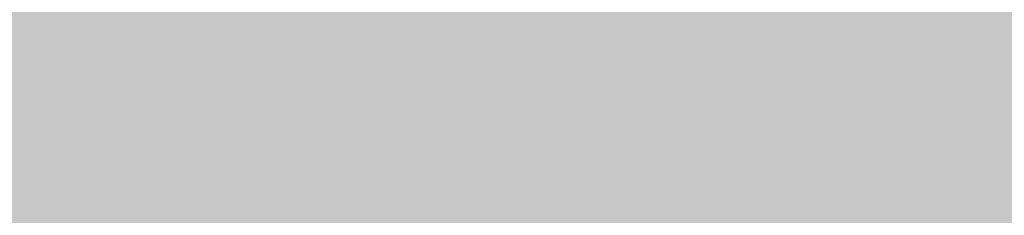
# Model space of a CAD drawing. Units: millimetres. Extents: x -22994 to 29398, y -19990 to 20176.
# Tile 92 of 135: x 229.428 to 230.597, y 83.564 to 83.796. Entities that reach past the tile are written whole.
import ezdxf
from ezdxf import colors
from ezdxf.entities.mleader import LeaderData, LeaderLine
from ezdxf.math import Vec2, Vec3

# ---------------------------------------------------------------- set-up
doc = ezdxf.new("R2010")
doc.units = ezdxf.units.MM
doc.header["$MEASUREMENT"] = 0
for name, color, linetype, lineweight in [('M-ANNO-TEXT', 7, 'Continuous', 25), ('M-DIMS', 2, 'Continuous', 18), ('M-EQPM-PATT', 7, 'Continuous', 18)]:
    doc.layers.add(name, color=color, linetype=linetype, lineweight=lineweight)
doc.styles.get("Standard").update_dxf_attribs({"font": 'arial.ttf'})
doc.dimstyles.get("Standard").update_dxf_attribs({"dimtxt": 0.18, "dimasz": 10000, "dimexe": 0.18, "dimexo": 0.0625, "dimgap": 0.09, "dimtad": 0, "dimtih": 1, "dimtoh": 1, "dimdec": 0, "dimzin": 0, "dimdsep": 46, "dimtxsty": 'Standard', "dimcen": 0.09, "dimadec": 0, "dimazin": 0, "dimtfac": 1, "dimtdec": 0, "dimtofl": 0, "dimtmove": 0, "dimatfit": 3, "dimfxl": 1, "dimtolj": 1, "dimtzin": 0, "dimlwd": 30, "dimarcsym": 0})

# ---------------------------------------------------------------- blocks, each defined once
blk = doc.blocks.new('*D2')
at = {"layer": 'Defpoints', "color": 0, "transparency": 16777216}
for p in [(6.6773, 10.2713), (290.852, 10.2713), (290.852, -5.0787)]:
    blk.add_point(p, dxfattribs=at)
at = {"layer": 'M-DIMS', "color": 0, "lineweight": -2, "transparency": 16777216}
for p, q in [((6.6773, 10.2088), (6.6773, -5.2587)), ((290.852, 10.2088), (290.852, -5.2587))]:
    blk.add_line(p, q, dxfattribs=at)
at = {"layer": 'M-DIMS', "color": 0, "lineweight": 30, "transparency": 16777216}
for p, q in [((-9993.3227, -5.0787), (-19993.3227, -5.0787)), ((10290.852, -5.0787), (20290.852, -5.0787))]:
    blk.add_line(p, q, dxfattribs=at)
at = {"layer": 'M-DIMS', "color": 0, "transparency": 16777216}
for points in [[(-9993.3227, 1661.5879), (-9993.3227, -1671.7454), (6.6773, -5.0787)], [(10290.852, 1661.5879), (10290.852, -1671.7454), (290.852, -5.0787)]]:
    blk.add_solid(points, dxfattribs=at)
at = {"layer": 'M-DIMS', "color": 0, "transparency": 16777216, "insert": (148.7647, -5.0787), "char_height": 0.18, "attachment_point": 5}
blk.add_mtext('\\A1;284.2', dxfattribs=at)
blk = doc.blocks.new('*D3')
at = {"layer": 'Defpoints', "color": 0, "transparency": 16777216}
for p in [(110.2647, 204.1654), (110.2647, 176.3662), (95.8327, 127.967)]:
    blk.add_point(p, dxfattribs=at)
at = {"layer": 'M-DIMS', "color": 0, "lineweight": -2, "transparency": 16777216}
for p, q in [((95.8327, 128.0295), (95.8327, 204.3454)), ((110.2647, 176.4287), (110.2647, 204.3454))]:
    blk.add_line(p, q, dxfattribs=at)
at = {"layer": 'M-DIMS', "color": 0, "lineweight": 30, "transparency": 16777216}
for p, q in [((-9904.1673, 204.1654), (-19904.1673, 204.1654)), ((10110.2647, 204.1654), (20110.2647, 204.1654))]:
    blk.add_line(p, q, dxfattribs=at)
at = {"layer": 'M-DIMS', "color": 0, "transparency": 16777216}
for points in [[(-9904.1673, 1870.8321), (-9904.1673, -1462.5013), (95.8327, 204.1654)], [(10110.2647, 1870.8321), (10110.2647, -1462.5013), (110.2647, 204.1654)]]:
    blk.add_solid(points, dxfattribs=at)
at = {"layer": 'M-DIMS', "color": 0, "transparency": 16777216, "insert": (103.0487, 204.1654), "char_height": 0.18, "attachment_point": 5}
blk.add_mtext('\\A1;14.432', dxfattribs=at)
blk = doc.blocks.new('*D4')
at = {"layer": 'Defpoints', "color": 0, "transparency": 16777216}
for p in [(116.2647, 204.1654), (110.2647, 176.3662), (116.2647, 176.3662)]:
    blk.add_point(p, dxfattribs=at)
at = {"layer": 'M-DIMS', "color": 0, "lineweight": -2, "transparency": 16777216}
for p, q in [((110.2647, 176.4287), (110.2647, 204.3454)), ((116.2647, 176.4287), (116.2647, 204.3454))]:
    blk.add_line(p, q, dxfattribs=at)
at = {"layer": 'M-DIMS', "color": 0, "lineweight": 30, "transparency": 16777216}
for p, q in [((-9889.7353, 204.1654), (-19889.7353, 204.1654)), ((10116.2647, 204.1654), (20116.2647, 204.1654))]:
    blk.add_line(p, q, dxfattribs=at)
at = {"layer": 'M-DIMS', "color": 0, "transparency": 16777216}
for points in [[(-9889.7353, 1870.8321), (-9889.7353, -1462.5013), (110.2647, 204.1654)], [(10116.2647, 1870.8321), (10116.2647, -1462.5013), (116.2647, 204.1654)]]:
    blk.add_solid(points, dxfattribs=at)
at = {"layer": 'M-DIMS', "color": 0, "transparency": 16777216, "insert": (113.2647, 204.1654), "char_height": 0.18, "attachment_point": 5}
blk.add_mtext('\\A1;6', dxfattribs=at)
blk = doc.blocks.new('*D5')
at = {"layer": 'Defpoints', "color": 0, "transparency": 16777216}
for p in [(181.2647, 204.1654), (116.2647, 176.3662), (181.2647, 176.3662)]:
    blk.add_point(p, dxfattribs=at)
at = {"layer": 'M-DIMS', "color": 0, "lineweight": -2, "transparency": 16777216}
for p, q in [((116.2647, 176.4287), (116.2647, 204.3454)), ((181.2647, 176.4287), (181.2647, 204.3454))]:
    blk.add_line(p, q, dxfattribs=at)
at = {"layer": 'M-DIMS', "color": 0, "lineweight": 30, "transparency": 16777216}
for p, q in [((-9883.7353, 204.1654), (-19883.7353, 204.1654)), ((10181.2647, 204.1654), (20181.2647, 204.1654))]:
    blk.add_line(p, q, dxfattribs=at)
at = {"layer": 'M-DIMS', "color": 0, "transparency": 16777216}
for points in [[(-9883.7353, 1870.8321), (-9883.7353, -1462.5013), (116.2647, 204.1654)], [(10181.2647, 1870.8321), (10181.2647, -1462.5013), (181.2647, 204.1654)]]:
    blk.add_solid(points, dxfattribs=at)
at = {"layer": 'M-DIMS', "color": 0, "transparency": 16777216, "insert": (148.7647, 204.1654), "char_height": 0.18, "attachment_point": 5}
blk.add_mtext('\\A1;65', dxfattribs=at)
blk = doc.blocks.new('*D6')
at = {"layer": 'Defpoints', "color": 0, "transparency": 16777216}
for p in [(187.2647, 204.1654), (181.2647, 176.3662), (187.2647, 176.3662)]:
    blk.add_point(p, dxfattribs=at)
at = {"layer": 'M-DIMS', "color": 0, "lineweight": -2, "transparency": 16777216}
for p, q in [((181.2647, 176.4287), (181.2647, 204.3454)), ((187.2647, 176.4287), (187.2647, 204.3454))]:
    blk.add_line(p, q, dxfattribs=at)
at = {"layer": 'M-DIMS', "color": 0, "lineweight": 30, "transparency": 16777216}
for p, q in [((-9818.7353, 204.1654), (-19818.7353, 204.1654)), ((10187.2647, 204.1654), (20187.2647, 204.1654))]:
    blk.add_line(p, q, dxfattribs=at)
at = {"layer": 'M-DIMS', "color": 0, "transparency": 16777216}
for points in [[(-9818.7353, 1870.8321), (-9818.7353, -1462.5013), (181.2647, 204.1654)], [(10187.2647, 1870.8321), (10187.2647, -1462.5013), (187.2647, 204.1654)]]:
    blk.add_solid(points, dxfattribs=at)
at = {"layer": 'M-DIMS', "color": 0, "transparency": 16777216, "insert": (184.2647, 204.1654), "char_height": 0.18, "attachment_point": 5}
blk.add_mtext('\\A1;6', dxfattribs=at)
blk = doc.blocks.new('*D7')
at = {"layer": 'Defpoints', "color": 0, "transparency": 16777216}
for p in [(201.6967, 204.1654), (187.2647, 176.3662), (201.6967, 127.967)]:
    blk.add_point(p, dxfattribs=at)
at = {"layer": 'M-DIMS', "color": 0, "lineweight": -2, "transparency": 16777216}
for p, q in [((187.2647, 176.4287), (187.2647, 204.3454)), ((201.6967, 128.0295), (201.6967, 204.3454))]:
    blk.add_line(p, q, dxfattribs=at)
at = {"layer": 'M-DIMS', "color": 0, "lineweight": 30, "transparency": 16777216}
for p, q in [((-9812.7353, 204.1654), (-19812.7353, 204.1654)), ((10201.6967, 204.1654), (20201.6967, 204.1654))]:
    blk.add_line(p, q, dxfattribs=at)
at = {"layer": 'M-DIMS', "color": 0, "transparency": 16777216}
for points in [[(-9812.7353, 1870.8321), (-9812.7353, -1462.5013), (187.2647, 204.1654)], [(10201.6967, 1870.8321), (10201.6967, -1462.5013), (201.6967, 204.1654)]]:
    blk.add_solid(points, dxfattribs=at)
at = {"layer": 'M-DIMS', "color": 0, "transparency": 16777216, "insert": (194.4807, 204.1654), "char_height": 0.18, "attachment_point": 5}
blk.add_mtext('\\A1;14.432', dxfattribs=at)
blk = doc.blocks.new('*D8')
at = {"layer": 'Defpoints', "color": 0, "transparency": 16777216}
for p in [(227.6485, 204.1654), (227.6485, 146.7296), (201.6967, 127.967)]:
    blk.add_point(p, dxfattribs=at)
at = {"layer": 'M-DIMS', "color": 0, "lineweight": -2, "transparency": 16777216}
for p, q in [((201.6967, 128.0295), (201.6967, 204.3454)), ((227.6485, 146.7921), (227.6485, 204.3454))]:
    blk.add_line(p, q, dxfattribs=at)
at = {"layer": 'M-DIMS', "color": 0, "lineweight": 30, "transparency": 16777216}
for p, q in [((-9798.3033, 204.1654), (-19798.3033, 204.1654)), ((10227.6485, 204.1654), (20227.6485, 204.1654))]:
    blk.add_line(p, q, dxfattribs=at)
at = {"layer": 'M-DIMS', "color": 0, "transparency": 16777216}
for points in [[(-9798.3033, 1870.8321), (-9798.3033, -1462.5013), (201.6967, 204.1654)], [(10227.6485, 1870.8321), (10227.6485, -1462.5013), (227.6485, 204.1654)]]:
    blk.add_solid(points, dxfattribs=at)
at = {"layer": 'M-DIMS', "color": 0, "transparency": 16777216, "insert": (214.6726, 204.1654), "char_height": 0.18, "attachment_point": 5}
blk.add_mtext('\\A1;25.95', dxfattribs=at)
blk = doc.blocks.new('*D9')
at = {"layer": 'Defpoints', "color": 0, "transparency": 16777216}
for p in [(187.2647, 176.3662), (306.202, 176.3662), (290.852, 10.2713)]:
    blk.add_point(p, dxfattribs=at)
at = {"layer": 'M-DIMS', "color": 0, "lineweight": 30, "transparency": 16777216}
for p, q in [((306.202, 10176.3662), (306.202, 20176.3662)), ((306.202, -9989.7287), (306.202, -19989.7287))]:
    blk.add_line(p, q, dxfattribs=at)
at = {"layer": 'M-DIMS', "color": 0, "lineweight": -2, "transparency": 16777216}
for p, q in [((187.3272, 176.3662), (306.382, 176.3662)), ((290.9145, 10.2713), (306.382, 10.2713))]:
    blk.add_line(p, q, dxfattribs=at)
at = {"layer": 'M-DIMS', "color": 0, "transparency": 16777216}
for points in [[(-1360.4646, 10176.3662), (1972.8687, 10176.3662), (306.202, 176.3662)], [(-1360.4646, -9989.7287), (1972.8687, -9989.7287), (306.202, 10.2713)]]:
    blk.add_solid(points, dxfattribs=at)
at = {"layer": 'M-DIMS', "color": 0, "transparency": 16777216, "insert": (306.202, 93.3187), "char_height": 0.18, "attachment_point": 5}
blk.add_mtext('\\A1;166.1', dxfattribs=at)
blk = doc.blocks.new('*D10')
at = {"layer": 'Defpoints', "color": 0, "transparency": 16777216}
for p in [(125.6498, 136.0713), (133.3459, 136.0713), (133.3459, -5.0787)]:
    blk.add_point(p, dxfattribs=at)
at = {"layer": 'M-DIMS', "color": 0, "lineweight": -2, "transparency": 16777216}
for p, q in [((125.6498, 136.0088), (125.6498, -5.2587)), ((133.3459, 136.0088), (133.3459, -5.2587))]:
    blk.add_line(p, q, dxfattribs=at)
at = {"layer": 'M-DIMS', "color": 0, "lineweight": 30, "transparency": 16777216}
for p, q in [((-9874.3502, -5.0787), (-19874.3502, -5.0787)), ((10133.3459, -5.0787), (20133.3459, -5.0787))]:
    blk.add_line(p, q, dxfattribs=at)
at = {"layer": 'M-DIMS', "color": 0, "transparency": 16777216}
for points in [[(-9874.3502, 1661.5879), (-9874.3502, -1671.7454), (125.6498, -5.0787)], [(10133.3459, 1661.5879), (10133.3459, -1671.7454), (133.3459, -5.0787)]]:
    blk.add_solid(points, dxfattribs=at)
at = {"layer": 'M-DIMS', "color": 0, "transparency": 16777216, "insert": (129.4978, -5.0787), "char_height": 0.18, "attachment_point": 5}
blk.add_mtext('\\A1;7.696', dxfattribs=at)
blk = doc.blocks.new('*D11')
at = {"layer": 'Defpoints', "color": 0, "transparency": 16777216}
for p in [(133.3459, 136.0713), (135.6498, 136.0713), (135.6498, -5.0787)]:
    blk.add_point(p, dxfattribs=at)
at = {"layer": 'M-DIMS', "color": 0, "lineweight": -2, "transparency": 16777216}
for p, q in [((133.3459, 136.0088), (133.3459, -5.2587)), ((135.6498, 136.0088), (135.6498, -5.2587))]:
    blk.add_line(p, q, dxfattribs=at)
at = {"layer": 'M-DIMS', "color": 0, "lineweight": 30, "transparency": 16777216}
for p, q in [((-9866.6541, -5.0787), (-19866.6541, -5.0787)), ((10135.6498, -5.0787), (20135.6498, -5.0787))]:
    blk.add_line(p, q, dxfattribs=at)
at = {"layer": 'M-DIMS', "color": 0, "transparency": 16777216}
for points in [[(-9866.6541, 1661.5879), (-9866.6541, -1671.7454), (133.3459, -5.0787)], [(10135.6498, 1661.5879), (10135.6498, -1671.7454), (135.6498, -5.0787)]]:
    blk.add_solid(points, dxfattribs=at)
at = {"layer": 'M-DIMS', "color": 0, "transparency": 16777216, "insert": (134.4978, -5.0787), "char_height": 0.18, "attachment_point": 5}
blk.add_mtext('\\A1;2.304', dxfattribs=at)
blk = doc.blocks.new('*D12')
at = {"layer": 'Defpoints', "color": 0, "transparency": 16777216}
for p in [(135.6498, 136.0713), (145.6498, 136.0713), (145.6498, -5.0787)]:
    blk.add_point(p, dxfattribs=at)
at = {"layer": 'M-DIMS', "color": 0, "lineweight": -2, "transparency": 16777216}
for p, q in [((135.6498, 136.0088), (135.6498, -5.2587)), ((145.6498, 136.0088), (145.6498, -5.2587))]:
    blk.add_line(p, q, dxfattribs=at)
at = {"layer": 'M-DIMS', "color": 0, "lineweight": 30, "transparency": 16777216}
for p, q in [((-9864.3502, -5.0787), (-19864.3502, -5.0787)), ((10145.6498, -5.0787), (20145.6498, -5.0787))]:
    blk.add_line(p, q, dxfattribs=at)
at = {"layer": 'M-DIMS', "color": 0, "transparency": 16777216}
for points in [[(-9864.3502, 1661.5879), (-9864.3502, -1671.7454), (135.6498, -5.0787)], [(10145.6498, 1661.5879), (10145.6498, -1671.7454), (145.6498, -5.0787)]]:
    blk.add_solid(points, dxfattribs=at)
at = {"layer": 'M-DIMS', "color": 0, "transparency": 16777216, "insert": (140.6498, -5.0787), "char_height": 0.18, "attachment_point": 5}
blk.add_mtext('\\A1;10', dxfattribs=at)
blk = doc.blocks.new('*D13')
at = {"layer": 'Defpoints', "color": 0, "transparency": 16777216}
for p in [(145.6498, 136.0713), (155.6498, 136.0713), (155.6498, -5.0787)]:
    blk.add_point(p, dxfattribs=at)
at = {"layer": 'M-DIMS', "color": 0, "lineweight": -2, "transparency": 16777216}
for p, q in [((145.6498, 136.0088), (145.6498, -5.2587)), ((155.6498, 136.0088), (155.6498, -5.2587))]:
    blk.add_line(p, q, dxfattribs=at)
at = {"layer": 'M-DIMS', "color": 0, "lineweight": 30, "transparency": 16777216}
for p, q in [((-9854.3502, -5.0787), (-19854.3502, -5.0787)), ((10155.6498, -5.0787), (20155.6498, -5.0787))]:
    blk.add_line(p, q, dxfattribs=at)
at = {"layer": 'M-DIMS', "color": 0, "transparency": 16777216}
for points in [[(-9854.3502, 1661.5879), (-9854.3502, -1671.7454), (145.6498, -5.0787)], [(10155.6498, 1661.5879), (10155.6498, -1671.7454), (155.6498, -5.0787)]]:
    blk.add_solid(points, dxfattribs=at)
at = {"layer": 'M-DIMS', "color": 0, "transparency": 16777216, "insert": (150.6498, -5.0787), "char_height": 0.18, "attachment_point": 5}
blk.add_mtext('\\A1;10', dxfattribs=at)
blk = doc.blocks.new('*D14')
at = {"layer": 'Defpoints', "color": 0, "transparency": 16777216}
for p in [(155.6498, 136.0713), (165.6498, 136.0713), (165.6498, -5.0787)]:
    blk.add_point(p, dxfattribs=at)
at = {"layer": 'M-DIMS', "color": 0, "lineweight": -2, "transparency": 16777216}
for p, q in [((155.6498, 136.0088), (155.6498, -5.2587)), ((165.6498, 136.0088), (165.6498, -5.2587))]:
    blk.add_line(p, q, dxfattribs=at)
at = {"layer": 'M-DIMS', "color": 0, "lineweight": 30, "transparency": 16777216}
for p, q in [((-9844.3502, -5.0787), (-19844.3502, -5.0787)), ((10165.6498, -5.0787), (20165.6498, -5.0787))]:
    blk.add_line(p, q, dxfattribs=at)
at = {"layer": 'M-DIMS', "color": 0, "transparency": 16777216}
for points in [[(-9844.3502, 1661.5879), (-9844.3502, -1671.7454), (155.6498, -5.0787)], [(10165.6498, 1661.5879), (10165.6498, -1671.7454), (165.6498, -5.0787)]]:
    blk.add_solid(points, dxfattribs=at)
at = {"layer": 'M-DIMS', "color": 0, "transparency": 16777216, "insert": (160.6498, -5.0787), "char_height": 0.18, "attachment_point": 5}
blk.add_mtext('\\A1;10', dxfattribs=at)
blk = doc.blocks.new('*D15')
at = {"layer": 'Defpoints', "color": 0, "transparency": 16777216}
for p in [(173.3459, 154.788), (173.3459, 136.0713), (306.202, 136.0713)]:
    blk.add_point(p, dxfattribs=at)
at = {"layer": 'M-DIMS', "color": 0, "lineweight": 30, "transparency": 16777216}
for p, q in [((306.202, 10154.788), (306.202, 20154.788)), ((306.202, -9863.9287), (306.202, -19863.9287))]:
    blk.add_line(p, q, dxfattribs=at)
at = {"layer": 'M-DIMS', "color": 0, "lineweight": -2, "transparency": 16777216}
for p, q in [((173.4084, 154.788), (306.382, 154.788)), ((173.4084, 136.0713), (306.382, 136.0713))]:
    blk.add_line(p, q, dxfattribs=at)
at = {"layer": 'M-DIMS', "color": 0, "transparency": 16777216}
for points in [[(-1360.4646, 10154.788), (1972.8687, 10154.788), (306.202, 154.788)], [(-1360.4646, -9863.9287), (1972.8687, -9863.9287), (306.202, 136.0713)]]:
    blk.add_solid(points, dxfattribs=at)
at = {"layer": 'M-DIMS', "color": 0, "transparency": 16777216, "insert": (306.202, 145.4297), "char_height": 0.18, "attachment_point": 5}
blk.add_mtext('\\A1;18.717', dxfattribs=at)
blk = doc.blocks.new('*D16')
at = {"layer": 'Defpoints', "color": 0, "transparency": 16777216}
for p in [(120.1702, 204.1654), (110.4658, 48.0349), (120.1702, 48.0349)]:
    blk.add_point(p, dxfattribs=at)
at = {"layer": 'M-DIMS', "color": 0, "lineweight": -2, "transparency": 16777216}
for p, q in [((110.4658, 48.0974), (110.4658, 204.3454)), ((120.1702, 48.0974), (120.1702, 204.3454))]:
    blk.add_line(p, q, dxfattribs=at)
at = {"layer": 'M-DIMS', "color": 0, "lineweight": 30, "transparency": 16777216}
for p, q in [((-9889.5342, 204.1654), (-19889.5342, 204.1654)), ((10120.1702, 204.1654), (20120.1702, 204.1654))]:
    blk.add_line(p, q, dxfattribs=at)
at = {"layer": 'M-DIMS', "color": 0, "transparency": 16777216}
for points in [[(-9889.5342, 1870.8321), (-9889.5342, -1462.5013), (110.4658, 204.1654)], [(10120.1702, 1870.8321), (10120.1702, -1462.5013), (120.1702, 204.1654)]]:
    blk.add_solid(points, dxfattribs=at)
at = {"layer": 'M-DIMS', "color": 0, "transparency": 16777216, "insert": (115.318, 204.1654), "char_height": 0.18, "attachment_point": 5}
blk.add_mtext('\\A1;9.704', dxfattribs=at)
blk = doc.blocks.new('*D17')
at = {"layer": 'Defpoints', "color": 0, "transparency": 16777216}
for p in [(126.1702, 204.1654), (120.1702, 48.0349), (126.1702, 48.0349)]:
    blk.add_point(p, dxfattribs=at)
at = {"layer": 'M-DIMS', "color": 0, "lineweight": -2, "transparency": 16777216}
for p, q in [((120.1702, 48.0974), (120.1702, 204.3454)), ((126.1702, 48.0974), (126.1702, 204.3454))]:
    blk.add_line(p, q, dxfattribs=at)
at = {"layer": 'M-DIMS', "color": 0, "lineweight": 30, "transparency": 16777216}
for p, q in [((-9879.8298, 204.1654), (-19879.8298, 204.1654)), ((10126.1702, 204.1654), (20126.1702, 204.1654))]:
    blk.add_line(p, q, dxfattribs=at)
at = {"layer": 'M-DIMS', "color": 0, "transparency": 16777216}
for points in [[(-9879.8298, 1870.8321), (-9879.8298, -1462.5013), (120.1702, 204.1654)], [(10126.1702, 1870.8321), (10126.1702, -1462.5013), (126.1702, 204.1654)]]:
    blk.add_solid(points, dxfattribs=at)
at = {"layer": 'M-DIMS', "color": 0, "transparency": 16777216, "insert": (123.1702, 204.1654), "char_height": 0.18, "attachment_point": 5}
blk.add_mtext('\\A1;6', dxfattribs=at)
blk = doc.blocks.new('*D18')
at = {"layer": 'Defpoints', "color": 0, "transparency": 16777216}
for p in [(132.1702, 204.1654), (126.1702, 48.0349), (132.1702, 48.0349)]:
    blk.add_point(p, dxfattribs=at)
at = {"layer": 'M-DIMS', "color": 0, "lineweight": -2, "transparency": 16777216}
for p, q in [((126.1702, 48.0974), (126.1702, 204.3454)), ((132.1702, 48.0974), (132.1702, 204.3454))]:
    blk.add_line(p, q, dxfattribs=at)
at = {"layer": 'M-DIMS', "color": 0, "lineweight": 30, "transparency": 16777216}
for p, q in [((-9873.8298, 204.1654), (-19873.8298, 204.1654)), ((10132.1702, 204.1654), (20132.1702, 204.1654))]:
    blk.add_line(p, q, dxfattribs=at)
at = {"layer": 'M-DIMS', "color": 0, "transparency": 16777216}
for points in [[(-9873.8298, 1870.8321), (-9873.8298, -1462.5013), (126.1702, 204.1654)], [(10132.1702, 1870.8321), (10132.1702, -1462.5013), (132.1702, 204.1654)]]:
    blk.add_solid(points, dxfattribs=at)
at = {"layer": 'M-DIMS', "color": 0, "transparency": 16777216, "insert": (129.1702, 204.1654), "char_height": 0.18, "attachment_point": 5}
blk.add_mtext('\\A1;6', dxfattribs=at)
blk = doc.blocks.new('*D19')
at = {"layer": 'Defpoints', "color": 0, "transparency": 16777216}
for p in [(138.1702, 204.1654), (132.1702, 48.0349), (138.1702, 48.0349)]:
    blk.add_point(p, dxfattribs=at)
at = {"layer": 'M-DIMS', "color": 0, "lineweight": -2, "transparency": 16777216}
for p, q in [((132.1702, 48.0974), (132.1702, 204.3454)), ((138.1702, 48.0974), (138.1702, 204.3454))]:
    blk.add_line(p, q, dxfattribs=at)
at = {"layer": 'M-DIMS', "color": 0, "lineweight": 30, "transparency": 16777216}
for p, q in [((-9867.8298, 204.1654), (-19867.8298, 204.1654)), ((10138.1702, 204.1654), (20138.1702, 204.1654))]:
    blk.add_line(p, q, dxfattribs=at)
at = {"layer": 'M-DIMS', "color": 0, "transparency": 16777216}
for points in [[(-9867.8298, 1870.8321), (-9867.8298, -1462.5013), (132.1702, 204.1654)], [(10138.1702, 1870.8321), (10138.1702, -1462.5013), (138.1702, 204.1654)]]:
    blk.add_solid(points, dxfattribs=at)
at = {"layer": 'M-DIMS', "color": 0, "transparency": 16777216, "insert": (135.1702, 204.1654), "char_height": 0.18, "attachment_point": 5}
blk.add_mtext('\\A1;6', dxfattribs=at)
blk = doc.blocks.new('*D20')
at = {"layer": 'Defpoints', "color": 0, "transparency": 16777216}
for p in [(144.1702, 204.1654), (138.1702, 48.0349), (144.1702, 48.0349)]:
    blk.add_point(p, dxfattribs=at)
at = {"layer": 'M-DIMS', "color": 0, "lineweight": -2, "transparency": 16777216}
for p, q in [((138.1702, 48.0974), (138.1702, 204.3454)), ((144.1702, 48.0974), (144.1702, 204.3454))]:
    blk.add_line(p, q, dxfattribs=at)
at = {"layer": 'M-DIMS', "color": 0, "lineweight": 30, "transparency": 16777216}
for p, q in [((-9861.8298, 204.1654), (-19861.8298, 204.1654)), ((10144.1702, 204.1654), (20144.1702, 204.1654))]:
    blk.add_line(p, q, dxfattribs=at)
at = {"layer": 'M-DIMS', "color": 0, "transparency": 16777216}
for points in [[(-9861.8298, 1870.8321), (-9861.8298, -1462.5013), (138.1702, 204.1654)], [(10144.1702, 1870.8321), (10144.1702, -1462.5013), (144.1702, 204.1654)]]:
    blk.add_solid(points, dxfattribs=at)
at = {"layer": 'M-DIMS', "color": 0, "transparency": 16777216, "insert": (141.1702, 204.1654), "char_height": 0.18, "attachment_point": 5}
blk.add_mtext('\\A1;6', dxfattribs=at)
blk = doc.blocks.new('*D21')
at = {"layer": 'Defpoints', "color": 0, "transparency": 16777216}
for p in [(149.1157, 204.1654), (144.1702, 48.0349), (149.1157, 48.0349)]:
    blk.add_point(p, dxfattribs=at)
at = {"layer": 'M-DIMS', "color": 0, "lineweight": -2, "transparency": 16777216}
for p, q in [((144.1702, 48.0974), (144.1702, 204.3454)), ((149.1157, 48.0974), (149.1157, 204.3454))]:
    blk.add_line(p, q, dxfattribs=at)
at = {"layer": 'M-DIMS', "color": 0, "lineweight": 30, "transparency": 16777216}
for p, q in [((-9855.8298, 204.1654), (-19855.8298, 204.1654)), ((10149.1157, 204.1654), (20149.1157, 204.1654))]:
    blk.add_line(p, q, dxfattribs=at)
at = {"layer": 'M-DIMS', "color": 0, "transparency": 16777216}
for points in [[(-9855.8298, 1870.8321), (-9855.8298, -1462.5013), (144.1702, 204.1654)], [(10149.1157, 1870.8321), (10149.1157, -1462.5013), (149.1157, 204.1654)]]:
    blk.add_solid(points, dxfattribs=at)
at = {"layer": 'M-DIMS', "color": 0, "transparency": 16777216, "insert": (146.6429, 204.1654), "char_height": 0.18, "attachment_point": 5}
blk.add_mtext('\\A1;4.945', dxfattribs=at)
blk = doc.blocks.new('*D22')
at = {"layer": 'Defpoints', "color": 0, "transparency": 16777216}
for p in [(149.1157, 30.9895), (155.1157, 30.9895), (155.1157, -5.0787)]:
    blk.add_point(p, dxfattribs=at)
at = {"layer": 'M-DIMS', "color": 0, "lineweight": -2, "transparency": 16777216}
for p, q in [((149.1157, 30.927), (149.1157, -5.2587)), ((155.1157, 30.927), (155.1157, -5.2587))]:
    blk.add_line(p, q, dxfattribs=at)
at = {"layer": 'M-DIMS', "color": 0, "lineweight": 30, "transparency": 16777216}
for p, q in [((-9850.8843, -5.0787), (-19850.8843, -5.0787)), ((10155.1157, -5.0787), (20155.1157, -5.0787))]:
    blk.add_line(p, q, dxfattribs=at)
at = {"layer": 'M-DIMS', "color": 0, "transparency": 16777216}
for points in [[(-9850.8843, 1661.5879), (-9850.8843, -1671.7454), (149.1157, -5.0787)], [(10155.1157, 1661.5879), (10155.1157, -1671.7454), (155.1157, -5.0787)]]:
    blk.add_solid(points, dxfattribs=at)
at = {"layer": 'M-DIMS', "color": 0, "transparency": 16777216, "insert": (152.1157, -5.0787), "char_height": 0.18, "attachment_point": 5}
blk.add_mtext('\\A1;6', dxfattribs=at)
blk = doc.blocks.new('*D23')
at = {"layer": 'Defpoints', "color": 0, "transparency": 16777216}
for p in [(155.1157, 30.9895), (161.1157, 30.9895), (161.1157, -5.0787)]:
    blk.add_point(p, dxfattribs=at)
at = {"layer": 'M-DIMS', "color": 0, "lineweight": -2, "transparency": 16777216}
for p, q in [((155.1157, 30.927), (155.1157, -5.2587)), ((161.1157, 30.927), (161.1157, -5.2587))]:
    blk.add_line(p, q, dxfattribs=at)
at = {"layer": 'M-DIMS', "color": 0, "lineweight": 30, "transparency": 16777216}
for p, q in [((-9844.8843, -5.0787), (-19844.8843, -5.0787)), ((10161.1157, -5.0787), (20161.1157, -5.0787))]:
    blk.add_line(p, q, dxfattribs=at)
at = {"layer": 'M-DIMS', "color": 0, "transparency": 16777216}
for points in [[(-9844.8843, 1661.5879), (-9844.8843, -1671.7454), (155.1157, -5.0787)], [(10161.1157, 1661.5879), (10161.1157, -1671.7454), (161.1157, -5.0787)]]:
    blk.add_solid(points, dxfattribs=at)
at = {"layer": 'M-DIMS', "color": 0, "transparency": 16777216, "insert": (158.1157, -5.0787), "char_height": 0.18, "attachment_point": 5}
blk.add_mtext('\\A1;6', dxfattribs=at)
blk = doc.blocks.new('*D24')
at = {"layer": 'Defpoints', "color": 0, "transparency": 16777216}
for p in [(161.1157, 30.9895), (166.4387, 30.9895), (166.4387, -5.0787)]:
    blk.add_point(p, dxfattribs=at)
at = {"layer": 'M-DIMS', "color": 0, "lineweight": -2, "transparency": 16777216}
for p, q in [((161.1157, 30.927), (161.1157, -5.2587)), ((166.4387, 30.927), (166.4387, -5.2587))]:
    blk.add_line(p, q, dxfattribs=at)
at = {"layer": 'M-DIMS', "color": 0, "lineweight": 30, "transparency": 16777216}
for p, q in [((-9838.8843, -5.0787), (-19838.8843, -5.0787)), ((10166.4387, -5.0787), (20166.4387, -5.0787))]:
    blk.add_line(p, q, dxfattribs=at)
at = {"layer": 'M-DIMS', "color": 0, "transparency": 16777216}
for points in [[(-9838.8843, 1661.5879), (-9838.8843, -1671.7454), (161.1157, -5.0787)], [(10166.4387, 1661.5879), (10166.4387, -1671.7454), (166.4387, -5.0787)]]:
    blk.add_solid(points, dxfattribs=at)
at = {"layer": 'M-DIMS', "color": 0, "transparency": 16777216, "insert": (163.7772, -5.0787), "char_height": 0.18, "attachment_point": 5}
blk.add_mtext('\\A1;5.323', dxfattribs=at)
blk = doc.blocks.new('*D25')
at = {"layer": 'Defpoints', "color": 0, "transparency": 16777216}
for p in [(166.4387, 30.9895), (172.4387, 30.9895), (172.4387, -5.0787)]:
    blk.add_point(p, dxfattribs=at)
at = {"layer": 'M-DIMS', "color": 0, "lineweight": -2, "transparency": 16777216}
for p, q in [((166.4387, 30.927), (166.4387, -5.2587)), ((172.4387, 30.927), (172.4387, -5.2587))]:
    blk.add_line(p, q, dxfattribs=at)
at = {"layer": 'M-DIMS', "color": 0, "lineweight": 30, "transparency": 16777216}
for p, q in [((-9833.5613, -5.0787), (-19833.5613, -5.0787)), ((10172.4387, -5.0787), (20172.4387, -5.0787))]:
    blk.add_line(p, q, dxfattribs=at)
at = {"layer": 'M-DIMS', "color": 0, "transparency": 16777216}
for points in [[(-9833.5613, 1661.5879), (-9833.5613, -1671.7454), (166.4387, -5.0787)], [(10172.4387, 1661.5879), (10172.4387, -1671.7454), (172.4387, -5.0787)]]:
    blk.add_solid(points, dxfattribs=at)
at = {"layer": 'M-DIMS', "color": 0, "transparency": 16777216, "insert": (169.4387, -5.0787), "char_height": 0.18, "attachment_point": 5}
blk.add_mtext('\\A1;6', dxfattribs=at)
blk = doc.blocks.new('*D26')
at = {"layer": 'Defpoints', "color": 0, "transparency": 16777216}
for p in [(172.4387, 30.9895), (178.4387, 30.9895), (178.4387, -5.0787)]:
    blk.add_point(p, dxfattribs=at)
at = {"layer": 'M-DIMS', "color": 0, "lineweight": -2, "transparency": 16777216}
for p, q in [((172.4387, 30.927), (172.4387, -5.2587)), ((178.4387, 30.927), (178.4387, -5.2587))]:
    blk.add_line(p, q, dxfattribs=at)
at = {"layer": 'M-DIMS', "color": 0, "lineweight": 30, "transparency": 16777216}
for p, q in [((-9827.5613, -5.0787), (-19827.5613, -5.0787)), ((10178.4387, -5.0787), (20178.4387, -5.0787))]:
    blk.add_line(p, q, dxfattribs=at)
at = {"layer": 'M-DIMS', "color": 0, "transparency": 16777216}
for points in [[(-9827.5613, 1661.5879), (-9827.5613, -1671.7454), (172.4387, -5.0787)], [(10178.4387, 1661.5879), (10178.4387, -1671.7454), (178.4387, -5.0787)]]:
    blk.add_solid(points, dxfattribs=at)
at = {"layer": 'M-DIMS', "color": 0, "transparency": 16777216, "insert": (175.4387, -5.0787), "char_height": 0.18, "attachment_point": 5}
blk.add_mtext('\\A1;6', dxfattribs=at)
blk = doc.blocks.new('*D27')
at = {"layer": 'Defpoints', "color": 0, "transparency": 16777216}
for p in [(178.4387, 30.9895), (188.1175, 30.9895), (188.1175, -5.0787)]:
    blk.add_point(p, dxfattribs=at)
at = {"layer": 'M-DIMS', "color": 0, "lineweight": -2, "transparency": 16777216}
for p, q in [((178.4387, 30.927), (178.4387, -5.2587)), ((188.1175, 30.927), (188.1175, -5.2587))]:
    blk.add_line(p, q, dxfattribs=at)
at = {"layer": 'M-DIMS', "color": 0, "lineweight": 30, "transparency": 16777216}
for p, q in [((-9821.5613, -5.0787), (-19821.5613, -5.0787)), ((10188.1175, -5.0787), (20188.1175, -5.0787))]:
    blk.add_line(p, q, dxfattribs=at)
at = {"layer": 'M-DIMS', "color": 0, "transparency": 16777216}
for points in [[(-9821.5613, 1661.5879), (-9821.5613, -1671.7454), (178.4387, -5.0787)], [(10188.1175, 1661.5879), (10188.1175, -1671.7454), (188.1175, -5.0787)]]:
    blk.add_solid(points, dxfattribs=at)
at = {"layer": 'M-DIMS', "color": 0, "transparency": 16777216, "insert": (183.2781, -5.0787), "char_height": 0.18, "attachment_point": 5}
blk.add_mtext('\\A1;9.679', dxfattribs=at)
blk = doc.blocks.new('*D28')
at = {"layer": 'Defpoints', "color": 0, "transparency": 16777216}
for p in [(188.1175, 48.0349), (306.202, 48.0349), (188.1175, 30.9895)]:
    blk.add_point(p, dxfattribs=at)
at = {"layer": 'M-DIMS', "color": 0, "lineweight": 30, "transparency": 16777216}
for p, q in [((306.202, 10048.0349), (306.202, 20048.0349)), ((306.202, -9969.0105), (306.202, -19969.0105))]:
    blk.add_line(p, q, dxfattribs=at)
at = {"layer": 'M-DIMS', "color": 0, "lineweight": -2, "transparency": 16777216}
for p, q in [((188.18, 48.0349), (306.382, 48.0349)), ((188.18, 30.9895), (306.382, 30.9895))]:
    blk.add_line(p, q, dxfattribs=at)
at = {"layer": 'M-DIMS', "color": 0, "transparency": 16777216}
for points in [[(-1360.4646, 10048.0349), (1972.8687, 10048.0349), (306.202, 48.0349)], [(-1360.4646, -9969.0105), (1972.8687, -9969.0105), (306.202, 30.9895)]]:
    blk.add_solid(points, dxfattribs=at)
at = {"layer": 'M-DIMS', "color": 0, "transparency": 16777216, "insert": (306.202, 39.5122), "char_height": 0.18, "attachment_point": 5}
blk.add_mtext('\\A1;17.045', dxfattribs=at)
blk = doc.blocks.new('*D29')
at = {"layer": 'Defpoints', "color": 0, "transparency": 16777216}
for p in [(36.8006, 80.045), (64.0296, 80.045)]:
    blk.add_point(p, dxfattribs=at)
at = {"layer": 'M-DIMS', "color": 0, "lineweight": -2, "transparency": 16777216}
for p, q in [((50.4151, 79.955), (50.4151, 80.135)), ((50.3251, 80.045), (50.5051, 80.045))]:
    blk.add_line(p, q, dxfattribs=at)
at = {"layer": 'M-DIMS', "color": 0, "lineweight": 30, "transparency": 16777216}
blk.add_line((20064.0296, 80.0303), (10064.0296, 80.0377), dxfattribs=at)
at = {"layer": 'M-DIMS', "color": 0, "transparency": 16777216}
blk.add_solid([(10064.0309, 1746.7043), (10064.0284, -1586.629), (64.0296, 80.045)], dxfattribs=at)
at = {"layer": 'M-DIMS', "color": 0, "transparency": 16777216, "insert": (20064.5213, 80.0303), "char_height": 0.18, "attachment_point": 5}
blk.add_mtext('\\A1;∅27.23', dxfattribs=at)
blk = doc.blocks.new('*D30')
at = {"layer": 'Defpoints', "color": 0, "transparency": 16777216}
for p in [(216.3148, 146.7291), (238.9821, 146.73)]:
    blk.add_point(p, dxfattribs=at)
at = {"layer": 'M-DIMS', "color": 0, "lineweight": 30, "transparency": 16777216}
blk.add_line((20238.9821, 147.4959), (10238.9821, 147.1129), dxfattribs=at)
at = {"layer": 'M-DIMS', "color": 0, "lineweight": -2, "transparency": 16777216}
for p, q in [((227.6485, 146.6396), (227.6485, 146.8196)), ((227.5585, 146.7296), (227.7385, 146.7296))]:
    blk.add_line(p, q, dxfattribs=at)
at = {"layer": 'M-DIMS', "color": 0, "transparency": 16777216}
blk.add_solid([(10238.9183, 1813.7796), (10239.0459, -1519.5537), (238.9821, 146.73)], dxfattribs=at)
at = {"layer": 'M-DIMS', "color": 0, "transparency": 16777216, "insert": (20239.5436, 147.4959), "char_height": 0.18, "attachment_point": 5}
blk.add_mtext('\\A1;∅22.667', dxfattribs=at)
blk = doc.blocks.new('*D31')
at = {"layer": 'Defpoints', "color": 0, "transparency": 16777216}
for p in [(223.1641, 146.7291), (232.1328, 146.73)]:
    blk.add_point(p, dxfattribs=at)
at = {"layer": 'M-DIMS', "color": 0, "lineweight": 30, "transparency": 16777216}
blk.add_line((20232.1327, 148.6656), (10232.1328, 147.6978), dxfattribs=at)
at = {"layer": 'M-DIMS', "color": 0, "lineweight": -2, "transparency": 16777216}
for p, q in [((227.6485, 146.6396), (227.6485, 146.8196)), ((227.5585, 146.7296), (227.7385, 146.7296))]:
    blk.add_line(p, q, dxfattribs=at)
at = {"layer": 'M-DIMS', "color": 0, "transparency": 16777216}
blk.add_solid([(10231.9715, 1814.3645), (10232.2941, -1518.9688), (232.1328, 146.73)], dxfattribs=at)
at = {"layer": 'M-DIMS', "color": 0, "transparency": 16777216, "insert": (20232.6245, 148.6656), "char_height": 0.18, "attachment_point": 5}
blk.add_mtext('\\A1;∅8.969', dxfattribs=at)
blk = doc.blocks.new('*D33')
at = {"layer": 'Defpoints', "color": 0, "transparency": 16777216}
for p in [(229.5613, 154.3773), (232.9972, 153.3509)]:
    blk.add_point(p, dxfattribs=at)
at = {"layer": 'M-DIMS', "color": 0, "lineweight": -2, "transparency": 16777216}
for p, q in [((229.5613, 154.2873), (229.5613, 154.4673)), ((229.4713, 154.3773), (229.6513, 154.3773))]:
    blk.add_line(p, q, dxfattribs=at)
at = {"layer": 'M-DIMS', "color": 0, "lineweight": 30, "transparency": 16777216}
for p, q in [((19396.3388, -5570.8378), (9814.668, -2708.7434)), ((29396.3388, -5570.8378), (19396.3388, -5570.8378))]:
    blk.add_line(p, q, dxfattribs=at)
at = {"layer": 'M-DIMS', "color": 0, "transparency": 16777216}
blk.add_solid([(10291.6837, -1111.7983), (9337.6523, -4305.6886), (232.9972, 153.3509)], dxfattribs=at)
at = {"layer": 'M-DIMS', "color": 0, "transparency": 16777216, "insert": (29397.0125, -5570.8378), "char_height": 0.18, "attachment_point": 5}
blk.add_mtext('\\A1;6X R3.586', dxfattribs=at)
blk = doc.blocks.new('*D36')
at = {"layer": 'Defpoints', "color": 0, "transparency": 16777216}
for p in [(46.39, 31.3035), (46.3875, 26.5934)]:
    blk.add_point(p, dxfattribs=at)
at = {"layer": 'M-DIMS', "color": 0, "lineweight": 30, "transparency": 16777216}
for p, q in [((57.1499, 20031.3006), (51.77, 10031.302)), ((10057.1499, 20031.3006), (57.1499, 20031.3006))]:
    blk.add_line(p, q, dxfattribs=at)
at = {"layer": 'M-DIMS', "color": 0, "lineweight": -2, "transparency": 16777216}
for p, q in [((46.3887, 28.8585), (46.3887, 29.0385)), ((46.2987, 28.9485), (46.4787, 28.9485))]:
    blk.add_line(p, q, dxfattribs=at)
at = {"layer": 'M-DIMS', "color": 0, "transparency": 16777216}
blk.add_solid([(-1614.8965, 10032.1987), (1718.4364, 10030.4054), (46.39, 31.3035)], dxfattribs=at)
at = {"layer": 'M-DIMS', "color": 0, "transparency": 16777216, "insert": (10057.5542, 20031.3006), "char_height": 0.18, "attachment_point": 5}
blk.add_mtext('\\A1;∅4.71', dxfattribs=at)

msp = doc.modelspace()

# ---------------------------------------------------------------- hatches: boundary and pattern name
at = {"layer": 'M-EQPM-PATT'}
h = msp.add_hatch(color=256, dxfattribs=at)
h.set_gradient(color1=(205, 32, 39), color2=(205, 32, 39), tint=1)
h.paths.add_polyline_path([(116.2647, 150.3662), (116.2647, 170.3662), (116.2647, 176.3662), (110.2647, 176.3662), (110.2647, 152.0276), (95.8327, 127.967), (95.8327, 16.6063), (201.6967, 16.6063), (201.6967, 127.967), (187.2647, 152.0276), (187.2647, 176.3662), (181.2647, 176.3662), (181.2647, 170.3662), (181.2647, 150.3662), (195.6967, 126.3055), (195.6967, 22.6063), (101.8327, 22.6063), (101.8327, 126.3055)])
h.paths.add_polyline_path([(185.2208, 88.6347), (101.8327, 88.6347), (101.8327, 87.6347), (182.8066, 87.6347), (178.7313, 83.5594), (195.6967, 83.5594), (195.6967, 84.5594), (181.1455, 84.5594)], flags=17)
h.paths.add_polyline_path([(95.8327, 88.6347), (60.9779, 88.6347, -0.022855), (61.7178, 87.6347), (95.8327, 87.6347)])
h.paths.add_polyline_path([(215.6212, 86.5189), (215.6212, 80.5999), (220.5095, 83.5594)])
h.paths.add_polyline_path([(215.6212, 84.5594), (201.6967, 84.5594), (201.6967, 83.5594), (215.6212, 83.5594)])
h.paths.add_polyline_path([(225.3978, 86.5189), (220.5095, 83.5594), (225.3978, 80.5999)])
h.paths.add_polyline_path([(231.6256, 84.5594), (225.3978, 84.5594), (225.3978, 83.5594), (231.6256, 83.5594)])

# ---------------------------------------------------------------- dimensions: what is measured, and where the dimension line sits
at = {"layer": 'M-DIMS'}
for base, p1, p2, override, picture, middle in [((306.202, 176.3662), (290.852, 10.2713), (187.2647, 176.3662), {"dimdec": 1, "dimlfac": 1, "dimrnd": 0, "dimzin": 0, "dimdsep": 46, "dimlunit": 2}, '*D9', (306.202, 93.3187)), ((306.202, 136.0713), (173.3459, 154.788), (173.3459, 136.0713), {"dimdec": 3, "dimlfac": 1, "dimrnd": 0, "dimzin": 0, "dimdsep": 46, "dimlunit": 2}, '*D15', (306.202, 145.4297)), ((306.202, 48.0349), (188.1175, 30.9895), (188.1175, 48.0349), {"dimdec": 3, "dimlfac": 1, "dimrnd": 0, "dimzin": 0, "dimdsep": 46, "dimlunit": 2}, '*D28', (306.202, 39.5122))]:
    dim = msp.add_linear_dim(base=base, p1=p1, p2=p2, angle=90, dimstyle='Standard', override=override, dxfattribs=at)
    dim.commit()
    dim.dimension.update_dxf_attribs({"geometry": picture, "text_midpoint": middle})
for p1, p2, override, picture, middle in [((46.3875, 26.5934), (46.39, 31.3035), {"dimdec": 2, "dimlfac": 1, "dimrnd": 0, "dimzin": 0, "dimdsep": 46, "dimlunit": 2}, '*D36', (10057.5542, 20031.3006)), ((223.1641, 146.7291), (232.1328, 146.73), {"dimdec": 3, "dimlfac": 1, "dimrnd": 0, "dimzin": 0, "dimdsep": 46, "dimlunit": 2}, '*D31', (20232.1327, 148.6656)), ((216.3148, 146.7291), (238.9821, 146.73), {"dimdec": 3, "dimlfac": 1, "dimrnd": 0, "dimzin": 0, "dimdsep": 46, "dimlunit": 2}, '*D30', (20238.9821, 147.4959))]:
    dim = msp.add_diameter_dim_2p(p1=p1, p2=p2, dimstyle='Standard', override=override, dxfattribs=at)
    dim.commit()
    dim.dimension.update_dxf_attribs({"geometry": picture, "text_midpoint": middle, "dimtype": 163})
for base, p1, p2, override, picture, middle in [((110.2647, 204.1654), (95.8327, 127.967), (110.2647, 176.3662), {"dimdec": 3, "dimlfac": 1, "dimrnd": 0, "dimzin": 0, "dimdsep": 46, "dimlunit": 2}, '*D3', (103.0487, 204.1654)), ((116.2647, 204.1654), (110.2647, 176.3662), (116.2647, 176.3662), {"dimdec": 0, "dimlfac": 1, "dimrnd": 0, "dimzin": 0, "dimdsep": 46, "dimlunit": 2}, '*D4', (113.2647, 204.1654)), ((120.1702, 204.1654), (110.4658, 48.0349), (120.1702, 48.0349), {"dimdec": 3, "dimlfac": 1, "dimrnd": 0, "dimzin": 0, "dimdsep": 46, "dimlunit": 2}, '*D16', (115.318, 204.1654)), ((181.2647, 204.1654), (116.2647, 176.3662), (181.2647, 176.3662), {"dimdec": 0, "dimlfac": 1, "dimrnd": 0, "dimzin": 0, "dimdsep": 46, "dimlunit": 2}, '*D5', (148.7647, 204.1654)), ((126.1702, 204.1654), (120.1702, 48.0349), (126.1702, 48.0349), {"dimdec": 0, "dimlfac": 1, "dimrnd": 0, "dimzin": 0, "dimdsep": 46, "dimlunit": 2}, '*D17', (123.1702, 204.1654)), ((132.1702, 204.1654), (126.1702, 48.0349), (132.1702, 48.0349), {"dimdec": 0, "dimlfac": 1, "dimrnd": 0, "dimzin": 0, "dimdsep": 46, "dimlunit": 2}, '*D18', (129.1702, 204.1654)), ((138.1702, 204.1654), (132.1702, 48.0349), (138.1702, 48.0349), {"dimdec": 0, "dimlfac": 1, "dimrnd": 0, "dimzin": 0, "dimdsep": 46, "dimlunit": 2}, '*D19', (135.1702, 204.1654)), ((144.1702, 204.1654), (138.1702, 48.0349), (144.1702, 48.0349), {"dimdec": 0, "dimlfac": 1, "dimrnd": 0, "dimzin": 0, "dimdsep": 46, "dimlunit": 2}, '*D20', (141.1702, 204.1654)), ((149.11567, 204.16539), (144.17023, 48.03494), (149.11567, 48.03494), {"dimdec": 3, "dimlfac": 1, "dimrnd": 0, "dimzin": 0, "dimdsep": 46, "dimlunit": 2}, '*D21', (146.64295, 204.16539)), ((187.2647, 204.1654), (181.2647, 176.3662), (187.2647, 176.3662), {"dimdec": 0, "dimlfac": 1, "dimrnd": 0, "dimzin": 0, "dimdsep": 46, "dimlunit": 2}, '*D6', (184.2647, 204.1654)), ((201.6967, 204.1654), (187.2647, 176.3662), (201.6967, 127.967), {"dimdec": 3, "dimlfac": 1, "dimrnd": 0, "dimzin": 0, "dimdsep": 46, "dimlunit": 2}, '*D7', (194.4807, 204.1654)), ((227.6485, 204.1654), (201.6967, 127.967), (227.6485, 146.7296), {"dimdec": 2, "dimlfac": 1, "dimrnd": 0, "dimzin": 0, "dimdsep": 46, "dimlunit": 2}, '*D8', (214.6726, 204.1654)), ((290.852, -5.0787), (6.6773, 10.2713), (290.852, 10.2713), {"dimdec": 1, "dimlfac": 1, "dimrnd": 0, "dimzin": 0, "dimdsep": 46, "dimlunit": 2}, '*D2', (148.7647, -5.0787)), ((133.3459, -5.0787), (125.6498, 136.0713), (133.3459, 136.0713), {"dimdec": 3, "dimlfac": 1, "dimrnd": 0, "dimzin": 0, "dimdsep": 46, "dimlunit": 2}, '*D10', (129.4978, -5.0787)), ((135.6498, -5.0787), (133.3459, 136.0713), (135.6498, 136.0713), {"dimdec": 3, "dimlfac": 1, "dimrnd": 0, "dimzin": 0, "dimdsep": 46, "dimlunit": 2}, '*D11', (134.4978, -5.0787)), ((145.6498, -5.0787), (135.6498, 136.0713), (145.6498, 136.0713), {"dimdec": 0, "dimlfac": 1, "dimrnd": 0, "dimzin": 0, "dimdsep": 46, "dimlunit": 2}, '*D12', (140.6498, -5.0787)), ((155.6498, -5.0787), (145.6498, 136.0713), (155.6498, 136.0713), {"dimdec": 0, "dimlfac": 1, "dimrnd": 0, "dimzin": 0, "dimdsep": 46, "dimlunit": 2}, '*D13', (150.6498, -5.0787)), ((155.1157, -5.0787), (149.1157, 30.9895), (155.1157, 30.9895), {"dimdec": 0, "dimlfac": 1, "dimrnd": 0, "dimzin": 0, "dimdsep": 46, "dimlunit": 2}, '*D22', (152.1157, -5.0787)), ((161.1157, -5.0787), (155.1157, 30.9895), (161.1157, 30.9895), {"dimdec": 0, "dimlfac": 1, "dimrnd": 0, "dimzin": 0, "dimdsep": 46, "dimlunit": 2}, '*D23', (158.1157, -5.0787)), ((165.6498, -5.0787), (155.6498, 136.0713), (165.6498, 136.0713), {"dimdec": 0, "dimlfac": 1, "dimrnd": 0, "dimzin": 0, "dimdsep": 46, "dimlunit": 2}, '*D14', (160.6498, -5.0787)), ((166.4387, -5.0787), (161.1157, 30.9895), (166.4387, 30.9895), {"dimdec": 3, "dimlfac": 1, "dimrnd": 0, "dimzin": 0, "dimdsep": 46, "dimlunit": 2}, '*D24', (163.7772, -5.0787)), ((172.4387, -5.0787), (166.4387, 30.9895), (172.4387, 30.9895), {"dimdec": 0, "dimlfac": 1, "dimrnd": 0, "dimzin": 0, "dimdsep": 46, "dimlunit": 2}, '*D25', (169.4387, -5.0787)), ((178.4387, -5.0787), (172.4387, 30.9895), (178.4387, 30.9895), {"dimdec": 0, "dimlfac": 1, "dimrnd": 0, "dimzin": 0, "dimdsep": 46, "dimlunit": 2}, '*D26', (175.4387, -5.0787)), ((188.1175, -5.0787), (178.4387, 30.9895), (188.1175, 30.9895), {"dimdec": 3, "dimlfac": 1, "dimrnd": 0, "dimzin": 0, "dimdsep": 46, "dimlunit": 2}, '*D27', (183.2781, -5.0787))]:
    dim = msp.add_linear_dim(base=base, p1=p1, p2=p2, dimstyle='Standard', override=override, dxfattribs=at)
    dim.commit()
    dim.dimension.update_dxf_attribs({"geometry": picture, "text_midpoint": middle})
dim = msp.add_diameter_dim_2p(p1=(36.8006, 80.045), p2=(64.0296, 80.045), dimstyle='Standard', override={"dimdec": 2, "dimlfac": 1, "dimrnd": 0, "dimzin": 0, "dimdsep": 46, "dimlunit": 2}, dxfattribs=at)
dim.commit()
dim.dimension.update_dxf_attribs({"geometry": '*D29', "text_midpoint": (20064.0296, 80.0303)})
dim = msp.add_radius_dim(center=(229.5613, 154.3773), mpoint=(232.9972, 153.3509), text='6X <>', dimstyle='Standard', override={"dimdec": 3, "dimlfac": 1, "dimrnd": 0, "dimzin": 0, "dimdsep": 46, "dimlunit": 2}, dxfattribs=at)
dim.commit()
dim.dimension.update_dxf_attribs({"geometry": '*D33', "text_midpoint": (29397.0125, -5570.8378)})

# ---------------------------------------------------------------- leaders
at = {"layer": 'M-ANNO-TEXT'}
ml = msp.add_multileader_mtext('Standard', dxfattribs=at)
ml.set_content('combustion chamber', color=256)
ml.set_leader_properties()
ml.build(insert=Vec2(0, 0))
ml.multileader.update_dxf_attribs({"dogleg_length": 0.36, "arrow_head_size": 200})
ctx = ml.context
ctx.base_point, ctx.char_height, ctx.arrow_head_size, ctx.landing_gap_size, ctx.plane_origin = Vec3(215.7321, 57.9149), 3, 200, 0.09, Vec3(189.1175, 57.9149)
notes = []
notes.append((ctx, [(0, (1, 1, 0), (215.3721, 57.9149), (1, 0), 0.36, [(0, [(189.1175, 57.9149)], 0, [])])]))
ctx.mtext.insert, ctx.mtext.flow_direction = Vec3(215.8221, 59.4394), 5
for ctx, leaders in notes:
    for number, flags, end, landing, length, lines in leaders:
        leader = LeaderData()
        leader.index, (leader.has_last_leader_line, leader.has_dogleg_vector, leader.attachment_direction) = number, flags
        leader.last_leader_point, leader.dogleg_vector, leader.dogleg_length = Vec3(end), Vec3(landing), length
        for number, points, colour, breaks in lines:
            line = LeaderLine()
            line.index, line.vertices, line.color, line.breaks = number, Vec3.list(points), colors.encode_raw_color(colour), breaks
            leader.lines.append(line)
        ctx.leaders.append(leader)

doc.saveas('drawing.dxf')
